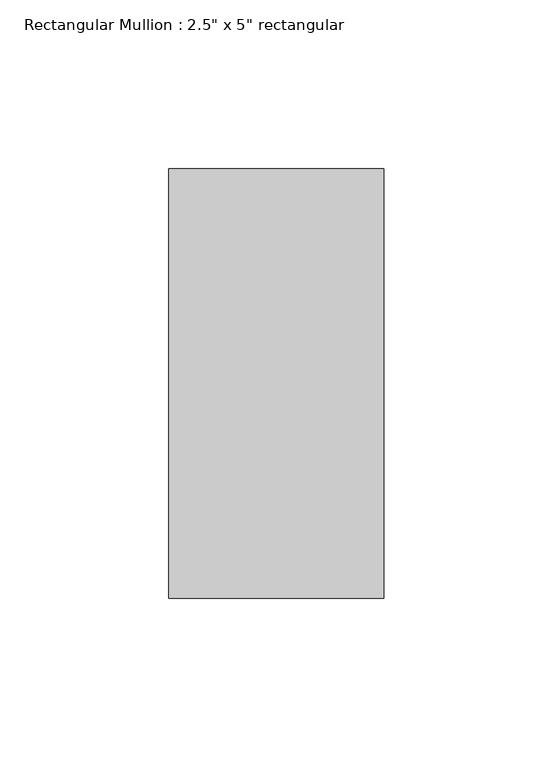
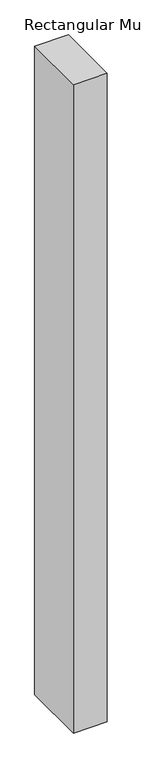
"""IFC4 building model written with IfcOpenShell, lengths in millimetres: member geometry."""

from ifc_helpers import new_model, si_unit, frame, origin, place, context, project, spatial, polyline, outline, extrude, source, transform, mapped, element, save


def member_efa17701(model_context):
    return source(origin(), model_context, "Body", "SweptSolid", [
        extrude(outline(polyline([(0.0, 63.5), (0.0, -63.5), (-63.5, -63.5), (-63.5, 63.5), (0.0, 63.5)])), frame((0.0, 0.0, -1294.4552325), z_axis=(0.0, 0.0, 1.0), x_axis=(1.0, 0.0, 0.0)), (0.0, 0.0, 1.0), 1294.4552325),
    ])


if __name__ == "__main__":
    model = new_model("IFC4")
    model_context = context("Model", 3, world=origin())
    ifc_project = project(units=[si_unit("LENGTHUNIT", "METRE", prefix="MILLI")], contexts=[model_context])
    site = spatial("IfcSite", under=ifc_project)
    building = spatial("IfcBuilding", under=site)
    placement = place(None, origin())
    member_shape = member_efa17701(model_context)
    element("IfcMember", 1, ObjectType="Rectangular Mullion : 2.5\" x 5\" rectangular", at=placement, inside=building, context=model_context, shape_type="MappedRepresentation", body=[
        mapped(member_shape, transform((0.0, 0.0, 0.0), x_axis=(1.0, 0.0, 0.0), y_axis=(0.0, 1.0, 0.0), z_axis=(0.0, 0.0, 1.0))),
    ])
    save(model, "model.ifc")

# Revit data of these elements
# Type "Rectangular Mullion : 2.5\" x 5\" rectangular"
#   built-in parameter 1007304 = 0.416667 (stored number, unit not read)
#   built-in parameter 1007301 = 0.104167 (stored number, unit not read)
#   built-in parameter 1007300 = 0.104167 (stored number, unit not read)
# Element 1 (IfcMember, "Rectangular Mullion : 2.5\" x 5\" rectangular")
#   Materials on its faces: "Iron, Ductile"
# Materials
#   "Iron, Ductile": class "Metal", colour RGB 0 0 0, transparency 0, Description = "Ductile cast iron", Cost = 0
